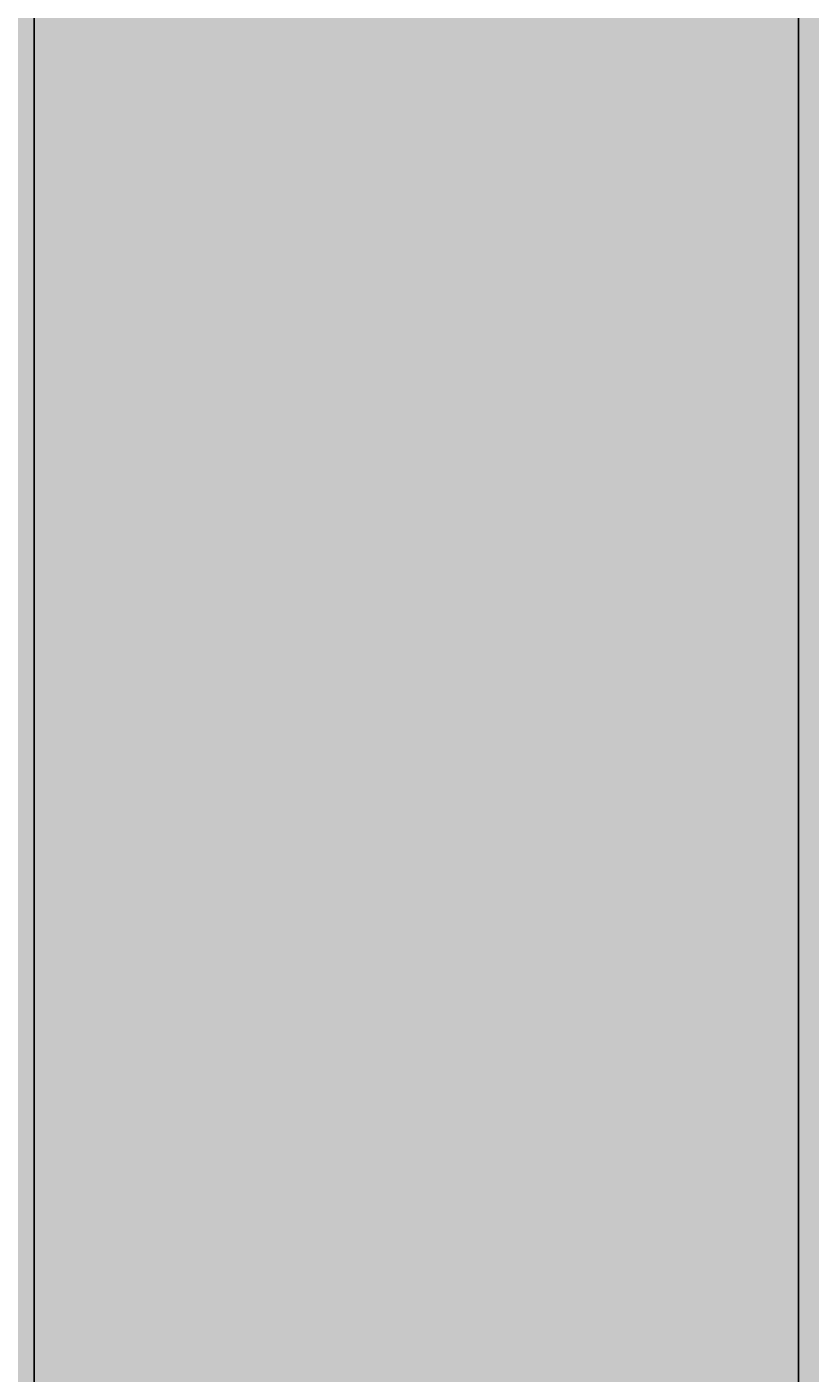
# Model space of a CAD drawing. Units: inches. Extents: x 4508 to 4723, y 847 to 1020.
# Tile 26 of 32: x 4631 to 4657, y 933 to 979. Entities that reach past the tile are written whole.
import ezdxf

# ---------------------------------------------------------------- set-up
doc = ezdxf.new("R2010")
doc.units = ezdxf.units.IN
doc.layers.add('A-ANNO-DIMS', color=2, linetype='Continuous', lineweight=18)
doc.layers.add('A-WALL-PATT', color=254, linetype='Continuous', lineweight=13)
doc.styles.get("Standard").update_dxf_attribs({"font": 'arial.ttf'})
doc.dimstyles.get("Standard").update_dxf_attribs({"dimtxt": 0.18, "dimasz": 0.18, "dimexe": 0.18, "dimexo": 0.0625, "dimgap": 0.09, "dimtad": 0, "dimtih": 1, "dimtoh": 1, "dimdec": 4, "dimzin": 0, "dimdsep": 46, "dimtxsty": 'Standard', "dimcen": 0.09, "dimadec": 0, "dimazin": 0, "dimtfac": 1, "dimtdec": 4, "dimtofl": 0, "dimtmove": 0, "dimatfit": 3, "dimfxl": 1, "dimtolj": 1, "dimtzin": 0, "dimarcsym": 0})

# ---------------------------------------------------------------- blocks, each defined once
blk = doc.blocks.new('*D7')
at = {"layer": 'A-ANNO-DIMS', "color": 0, "lineweight": -2, "transparency": 16777216}
for p, q in [((4588.994, 994.809), (4588.994, 1002.877)), ((4589.174, 1002.697), (4625.189, 1002.697)), ((4661.991, 1002.697), (4625.975, 1002.697)), ((4662.171, 957.665), (4662.171, 1002.877))]:
    blk.add_line(p, q, dxfattribs=at)
at = {"layer": 'A-ANNO-DIMS', "color": 0, "lineweight": 9, "transparency": 16777216}
for points in [[(4589.174, 1002.727), (4589.174, 1002.667), (4588.994, 1002.697)], [(4661.991, 1002.727), (4661.991, 1002.667), (4662.171, 1002.697)]]:
    blk.add_solid(points, dxfattribs=at)
at = {"layer": 'Defpoints', "color": 0, "lineweight": 9, "transparency": 16777216}
for p in [(4662.171, 1002.697), (4588.994, 994.747), (4662.171, 957.602)]:
    blk.add_point(p, dxfattribs=at)
at = {"layer": 'A-ANNO-DIMS', "color": 0, "transparency": 16777216, "insert": (4625.582, 1002.697), "char_height": 0.18, "attachment_point": 5}
blk.add_mtext('\\A1;73.18', dxfattribs=at)
blk = doc.blocks.new('*D31')
at = {"layer": 'A-ANNO-DIMS', "color": 0, "lineweight": -2, "transparency": 16777216}
for p, q in [((4630.994, 903.809), (4630.994, 1002.877)), ((4631.174, 1002.697), (4643.773, 1002.697)), ((4656.814, 1002.697), (4644.214, 1002.697)), ((4656.994, 903.809), (4656.994, 1002.877))]:
    blk.add_line(p, q, dxfattribs=at)
at = {"layer": 'A-ANNO-DIMS', "color": 0, "lineweight": 9, "transparency": 16777216}
for points in [[(4631.174, 1002.727), (4631.174, 1002.667), (4630.994, 1002.697)], [(4656.814, 1002.727), (4656.814, 1002.667), (4656.994, 1002.697)]]:
    blk.add_solid(points, dxfattribs=at)
at = {"layer": 'Defpoints', "color": 0, "lineweight": 9, "transparency": 16777216}
for p in [(4656.994, 1002.697), (4630.994, 903.747), (4656.994, 903.747)]:
    blk.add_point(p, dxfattribs=at)
at = {"layer": 'A-ANNO-DIMS', "color": 0, "transparency": 16777216, "insert": (4643.994, 1002.697), "char_height": 0.18, "attachment_point": 5}
blk.add_mtext('\\A1;26', dxfattribs=at)

msp = doc.modelspace()

# ---------------------------------------------------------------- hatches: boundary and pattern name
at = {"layer": 'A-WALL-PATT', "transparency": 33554508}
h = msp.add_hatch(color=256, dxfattribs=at)
h.dxf.hatch_style = 1
h.paths.add_polyline_path([(4661.6706, 954.043, -0.3739004), (4658.5765, 957.6021, -1), (4665.7646, 957.6021, -0.3739004), (4662.6706, 954.043), (4662.6706, 944.4021, -0.2114781), (4670.3062, 945.0869), (4670.3062, 968.0592, -0.4632086), (4663.3246, 973.9783, -0.4632086), (4670.3062, 979.8975), (4670.3062, 994.7469), (4588.9938, 994.7469), (4588.9938, 904.7469), (4657.9938, 904.7469), (4657.9938, 886.7469), (4549.9938, 886.7469), (4549.9938, 878.7469), (4693.9938, 878.7469), (4693.9938, 994.7469), (4671.8062, 994.7469), (4671.8062, 979.4411, -0.2941682), (4675.3246, 973.9783, -0.2941682), (4671.8062, 968.5156), (4671.8062, 944.4278, -0.2741114), (4676.7298, 936.1217, -0.2741114), (4671.8062, 927.8155), (4671.8062, 907.6998, -0.3779645), (4677.0562, 901.7469, -0.3779645), (4671.8062, 895.7939), (4671.8062, 883.7469), (4670.3062, 883.7469), (4670.3062, 895.7939, -0.3779645), (4665.0562, 901.7469, -0.3779645), (4670.3062, 907.6998), (4670.3062, 927.1564, -0.2114781), (4662.6706, 927.8412), (4662.6706, 918.2003, -0.3739004), (4665.7646, 914.6412, -1), (4658.5765, 914.6412, -0.3739004), (4661.6706, 918.2003), (4661.6706, 928.4807, -0.2391825), (4657.7936, 936.1217, -0.2391825), (4661.6706, 943.7626)])

# ---------------------------------------------------------------- dimensions: what is measured, and where the dimension line sits
at = {"layer": 'A-ANNO-DIMS'}
for base, p1, p2, override, picture, middle in [((4662.1706, 1002.6969), (4588.9938, 994.7469), (4662.1706, 957.6021), {"dimdec": 2, "dimlfac": 1, "dimrnd": 0, "dimzin": 0, "dimdsep": 46, "dimlunit": 2}, '*D7', (4625.5822, 1002.6969)), ((4656.9938, 1002.6969), (4630.9938, 903.7469), (4656.9938, 903.7469), {"dimdec": 0, "dimlfac": 1, "dimrnd": 0, "dimzin": 0, "dimdsep": 46, "dimlunit": 2}, '*D31', (4643.9938, 1002.6969))]:
    dim = msp.add_linear_dim(base=base, p1=p1, p2=p2, dimstyle='Standard', override=override, dxfattribs=at)
    dim.commit()
    dim.dimension.update_dxf_attribs({"geometry": picture, "text_midpoint": middle})

doc.saveas('drawing.dxf')
